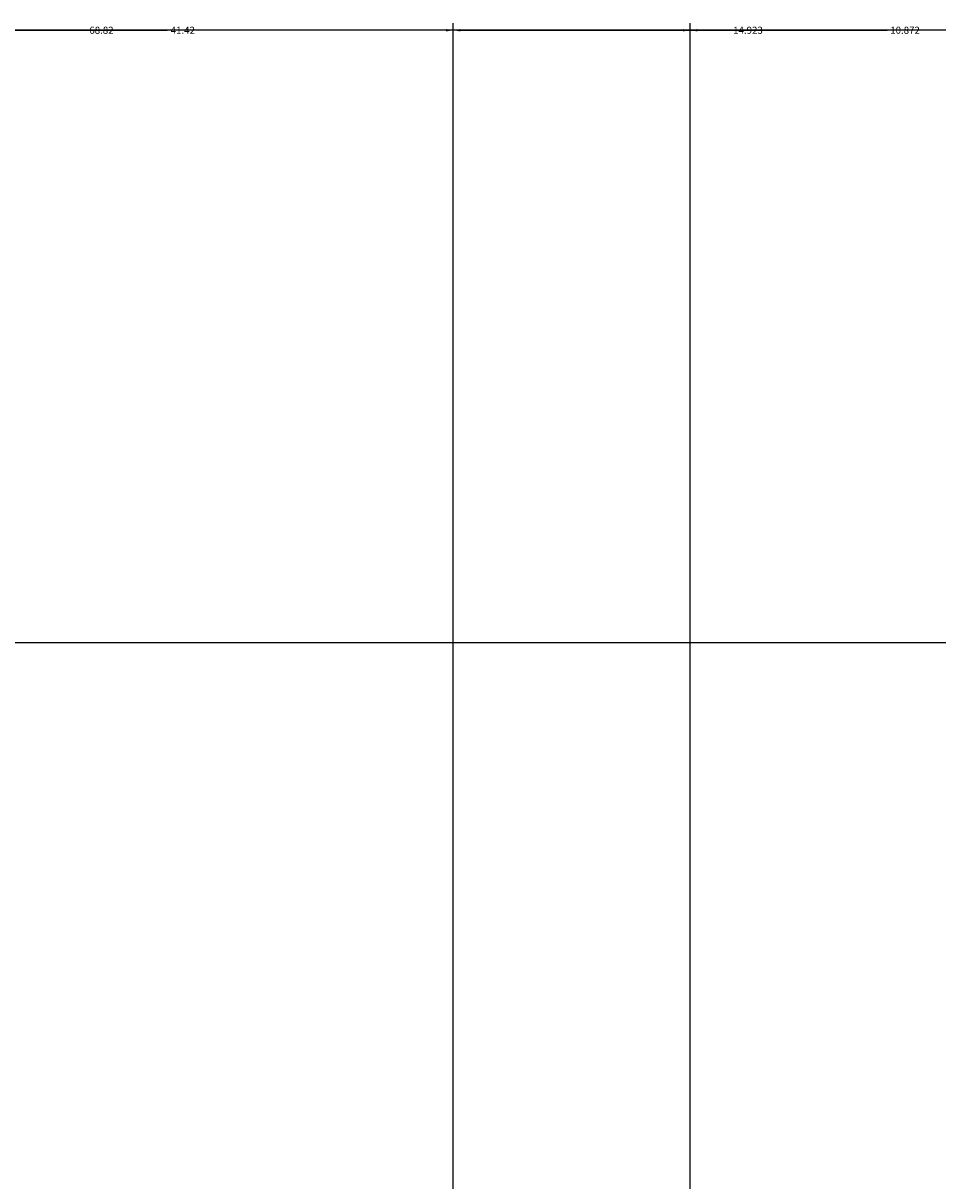
# Model space of a CAD drawing. Units: inches. Extents: x -6 to 289, y -8 to 323.
# Tile 103 of 107: x 219 to 243, y 294 to 323. Entities that reach past the tile are written whole.
import ezdxf

# ---------------------------------------------------------------- set-up
doc = ezdxf.new("R2010")
doc.units = ezdxf.units.IN
doc.header["$MEASUREMENT"] = 0
doc.layers.add('A-ANNO-DIMS', color=2, linetype='Continuous', lineweight=18)
doc.styles.get("Standard").update_dxf_attribs({"font": 'arial.ttf'})
doc.dimstyles.get("Standard").update_dxf_attribs({"dimtxt": 0.18, "dimasz": 0.18, "dimexe": 0.18, "dimexo": 0.0625, "dimgap": 0.09, "dimtad": 0, "dimtih": 1, "dimtoh": 1, "dimdec": 4, "dimzin": 0, "dimdsep": 46, "dimtxsty": 'Standard', "dimcen": 0.09, "dimadec": 0, "dimazin": 0, "dimtfac": 1, "dimtdec": 4, "dimtofl": 0, "dimtmove": 0, "dimatfit": 3, "dimfxl": 1, "dimtolj": 1, "dimtzin": 0, "dimarcsym": 0})

# ---------------------------------------------------------------- blocks, each defined once
blk = doc.blocks.new('*D13')
at = {"layer": 'A-ANNO-DIMS', "color": 0, "lineweight": -2, "transparency": 16777216}
for p, q in [((188.292, 226.951), (188.292, 322.969)), ((236.292, 226.951), (236.292, 322.969)), ((188.472, 322.789), (212.069, 322.789)), ((236.112, 322.789), (212.515, 322.789))]:
    blk.add_line(p, q, dxfattribs=at)
at = {"layer": 'A-ANNO-DIMS', "color": 0, "transparency": 16777216}
for points in [[(188.472, 322.819), (188.472, 322.759), (188.292, 322.789)], [(236.112, 322.819), (236.112, 322.759), (236.292, 322.789)]]:
    blk.add_solid(points, dxfattribs=at)
at = {"layer": 'Defpoints', "color": 0, "transparency": 16777216}
for p in [(236.292, 322.789), (188.292, 226.889), (236.292, 226.889)]:
    blk.add_point(p, dxfattribs=at)
at = {"layer": 'A-ANNO-DIMS', "color": 0, "transparency": 16777216, "insert": (212.292, 322.789), "char_height": 0.18, "attachment_point": 5}
blk.add_mtext('\\A1;48', dxfattribs=at)
blk = doc.blocks.new('*D14')
at = {"layer": 'A-ANNO-DIMS', "color": 0, "lineweight": -2, "transparency": 16777216}
for p, q in [((236.292, 226.951), (236.292, 322.969)), ((247.164, 162.411), (247.164, 322.969)), ((236.472, 322.789), (241.274, 322.789)), ((246.984, 322.789), (242.182, 322.789))]:
    blk.add_line(p, q, dxfattribs=at)
at = {"layer": 'A-ANNO-DIMS', "color": 0, "transparency": 16777216}
for points in [[(236.472, 322.819), (236.472, 322.759), (236.292, 322.789)], [(246.984, 322.819), (246.984, 322.759), (247.164, 322.789)]]:
    blk.add_solid(points, dxfattribs=at)
at = {"layer": 'Defpoints', "color": 0, "transparency": 16777216}
for p in [(247.164, 322.789), (236.292, 226.889), (247.164, 162.348)]:
    blk.add_point(p, dxfattribs=at)
at = {"layer": 'A-ANNO-DIMS', "color": 0, "transparency": 16777216, "insert": (241.728, 322.789), "char_height": 0.18, "attachment_point": 5}
blk.add_mtext('\\A1;10.872', dxfattribs=at)
blk = doc.blocks.new('*D27')
at = {"layer": 'A-ANNO-DIMS', "color": 0, "lineweight": -2, "transparency": 16777216}
for p, q in [((19.226, 307.289), (288.653, 307.289)), ((288.473, 307.109), (288.473, 277.471)), ((288.473, 247.469), (288.473, 277.107)), ((247.226, 247.289), (288.653, 247.289))]:
    blk.add_line(p, q, dxfattribs=at)
at = {"layer": 'A-ANNO-DIMS', "color": 0, "transparency": 16777216}
for points in [[(288.443, 307.109), (288.503, 307.109), (288.473, 307.289)], [(288.443, 247.469), (288.503, 247.469), (288.473, 247.289)]]:
    blk.add_solid(points, dxfattribs=at)
at = {"layer": 'Defpoints', "color": 0, "transparency": 16777216}
for p in [(19.164, 307.289), (288.473, 307.289), (247.164, 247.289)]:
    blk.add_point(p, dxfattribs=at)
at = {"layer": 'A-ANNO-DIMS', "color": 0, "transparency": 16777216, "insert": (288.473, 277.289), "char_height": 0.18, "attachment_point": 5}
blk.add_mtext('\\A1;60', dxfattribs=at)
blk = doc.blocks.new('*D80')
at = {"layer": 'A-ANNO-DIMS', "color": 0, "lineweight": -2, "transparency": 16777216}
for p, q in [((188.292, 116.842), (188.292, 322.969)), ((230.292, 116.842), (230.292, 322.969)), ((188.472, 322.789), (209.07, 322.789)), ((230.112, 322.789), (209.513, 322.789))]:
    blk.add_line(p, q, dxfattribs=at)
at = {"layer": 'A-ANNO-DIMS', "color": 0, "transparency": 16777216}
for points in [[(188.472, 322.819), (188.472, 322.759), (188.292, 322.789)], [(230.112, 322.819), (230.112, 322.759), (230.292, 322.789)]]:
    blk.add_solid(points, dxfattribs=at)
at = {"layer": 'Defpoints', "color": 0, "transparency": 16777216}
for p in [(230.292, 322.789), (188.292, 116.779), (230.292, 116.779)]:
    blk.add_point(p, dxfattribs=at)
at = {"layer": 'A-ANNO-DIMS', "color": 0, "transparency": 16777216, "insert": (209.292, 322.789), "char_height": 0.18, "attachment_point": 5}
blk.add_mtext('\\A1;42', dxfattribs=at)
blk = doc.blocks.new('*D81')
at = {"layer": 'A-ANNO-DIMS', "color": 0, "lineweight": -2, "transparency": 16777216}
for p, q in [((230.292, 68.842), (230.292, 322.969)), ((245.215, 66.286), (245.215, 322.969)), ((230.472, 322.789), (237.298, 322.789)), ((245.035, 322.789), (238.208, 322.789))]:
    blk.add_line(p, q, dxfattribs=at)
at = {"layer": 'A-ANNO-DIMS', "color": 0, "transparency": 16777216}
for points in [[(230.472, 322.819), (230.472, 322.759), (230.292, 322.789)], [(245.035, 322.819), (245.035, 322.759), (245.215, 322.789)]]:
    blk.add_solid(points, dxfattribs=at)
at = {"layer": 'Defpoints', "color": 0, "transparency": 16777216}
for p in [(245.215, 322.789), (230.292, 68.779), (245.215, 66.224)]:
    blk.add_point(p, dxfattribs=at)
at = {"layer": 'A-ANNO-DIMS', "color": 0, "transparency": 16777216, "insert": (237.753, 322.789), "char_height": 0.18, "attachment_point": 5}
blk.add_mtext('\\A1;14.923', dxfattribs=at)
blk = doc.blocks.new('*D98')
at = {"layer": 'A-ANNO-DIMS', "color": 0, "lineweight": -2, "transparency": 16777216}
for p, q in [((202.741, 159.411), (202.741, 322.969)), ((244.164, 159.411), (244.164, 322.969)), ((202.921, 322.789), (223.056, 322.789)), ((243.984, 322.789), (223.849, 322.789))]:
    blk.add_line(p, q, dxfattribs=at)
at = {"layer": 'A-ANNO-DIMS', "color": 0, "transparency": 16777216}
for points in [[(202.921, 322.819), (202.921, 322.759), (202.741, 322.789)], [(243.984, 322.819), (243.984, 322.759), (244.164, 322.789)]]:
    blk.add_solid(points, dxfattribs=at)
at = {"layer": 'Defpoints', "color": 0, "transparency": 16777216}
for p in [(244.164, 322.789), (202.741, 159.348), (244.164, 159.348)]:
    blk.add_point(p, dxfattribs=at)
at = {"layer": 'A-ANNO-DIMS', "color": 0, "transparency": 16777216, "insert": (223.452, 322.789), "char_height": 0.18, "attachment_point": 5}
blk.add_mtext('\\A1;41.42', dxfattribs=at)
blk = doc.blocks.new('*D108')
at = {"layer": 'A-ANNO-DIMS', "color": 0, "lineweight": -2, "transparency": 16777216}
for p, q in [((186.984, 291.541), (186.984, 322.969)), ((255.804, 291.541), (255.804, 322.969)), ((187.164, 322.789), (221, 322.789)), ((255.624, 322.789), (221.787, 322.789))]:
    blk.add_line(p, q, dxfattribs=at)
at = {"layer": 'A-ANNO-DIMS', "color": 0, "transparency": 16777216}
for points in [[(187.164, 322.819), (187.164, 322.759), (186.984, 322.789)], [(255.624, 322.819), (255.624, 322.759), (255.804, 322.789)]]:
    blk.add_solid(points, dxfattribs=at)
at = {"layer": 'Defpoints', "color": 0, "transparency": 16777216}
for p in [(255.804, 322.789), (186.984, 291.478), (255.804, 291.478)]:
    blk.add_point(p, dxfattribs=at)
at = {"layer": 'A-ANNO-DIMS', "color": 0, "transparency": 16777216, "insert": (221.394, 322.789), "char_height": 0.18, "attachment_point": 5}
blk.add_mtext('\\A1;68.82', dxfattribs=at)
blk = doc.blocks.new('*D118')
at = {"layer": 'A-ANNO-DIMS', "color": 0, "lineweight": -2, "transparency": 16777216}
for p, q in [((118.226, 307.289), (288.653, 307.289)), ((288.473, 307.109), (288.473, 300.659)), ((288.473, 293.846), (288.473, 300.295)), ((257.703, 293.666), (288.653, 293.666))]:
    blk.add_line(p, q, dxfattribs=at)
at = {"layer": 'A-ANNO-DIMS', "color": 0, "transparency": 16777216}
for points in [[(288.443, 307.109), (288.503, 307.109), (288.473, 307.289)], [(288.443, 293.846), (288.503, 293.846), (288.473, 293.666)]]:
    blk.add_solid(points, dxfattribs=at)
at = {"layer": 'Defpoints', "color": 0, "transparency": 16777216}
for p in [(118.164, 307.289), (288.473, 307.289), (257.641, 293.666)]:
    blk.add_point(p, dxfattribs=at)
at = {"layer": 'A-ANNO-DIMS', "color": 0, "transparency": 16777216, "insert": (288.473, 300.477), "char_height": 0.18, "attachment_point": 5}
blk.add_mtext('\\A1;13.623', dxfattribs=at)

msp = doc.modelspace()

# ---------------------------------------------------------------- dimensions: what is measured, and where the dimension line sits
at = {"layer": 'A-ANNO-DIMS'}
for base, p1, p2, override, picture, middle in [((255.8036, 322.7888), (186.9837, 291.4781), (255.8036, 291.4781), {"dimdec": 2, "dimlfac": 1, "dimrnd": 0, "dimzin": 0, "dimdsep": 46, "dimlunit": 2}, '*D108', (221.3936, 322.7888)), ((236.2918, 322.7888), (188.2918, 226.8887), (236.2918, 226.8887), {"dimdec": 0, "dimlfac": 1, "dimrnd": 0, "dimzin": 0, "dimdsep": 46, "dimlunit": 2}, '*D13', (212.2918, 322.7888)), ((230.2918, 322.7888), (188.2918, 116.7795), (230.2918, 116.7795), {"dimdec": 0, "dimlfac": 1, "dimrnd": 0, "dimzin": 0, "dimdsep": 46, "dimlunit": 2}, '*D80', (209.2918, 322.7888)), ((244.1638, 322.7888), (202.741, 159.3484), (244.1638, 159.3484), {"dimdec": 2, "dimlfac": 1, "dimrnd": 0, "dimzin": 0, "dimdsep": 46, "dimlunit": 2}, '*D98', (223.4524, 322.7888)), ((245.2146, 322.7888), (230.2918, 68.7795), (245.2146, 66.2238), {"dimdec": 3, "dimlfac": 1, "dimrnd": 0, "dimzin": 0, "dimdsep": 46, "dimlunit": 2}, '*D81', (237.7532, 322.7888)), ((247.1638, 322.7888), (236.2918, 226.8887), (247.1638, 162.3484), {"dimdec": 3, "dimlfac": 1, "dimrnd": 0, "dimzin": 0, "dimdsep": 46, "dimlunit": 2}, '*D14', (241.7278, 322.7888))]:
    dim = msp.add_linear_dim(base=base, p1=p1, p2=p2, dimstyle='Standard', override=override, dxfattribs=at)
    dim.commit()
    dim.dimension.update_dxf_attribs({"geometry": picture, "text_midpoint": middle})
for p1, p2, override, picture, middle in [((247.1638, 247.2888), (19.1638, 307.2888), {"dimdec": 0, "dimlfac": 1, "dimrnd": 0, "dimzin": 0, "dimdsep": 46, "dimlunit": 2}, '*D27', (288.4733, 277.2888)), ((257.6407, 293.6657), (118.1638, 307.2888), {"dimdec": 3, "dimlfac": 1, "dimrnd": 0, "dimzin": 0, "dimdsep": 46, "dimlunit": 2}, '*D118', (288.4733, 300.4773))]:
    dim = msp.add_linear_dim(base=(288.4733, 307.2888), p1=p1, p2=p2, angle=90, dimstyle='Standard', override=override, dxfattribs=at)
    dim.commit()
    dim.dimension.update_dxf_attribs({"geometry": picture, "text_midpoint": middle})

doc.saveas('drawing.dxf')
